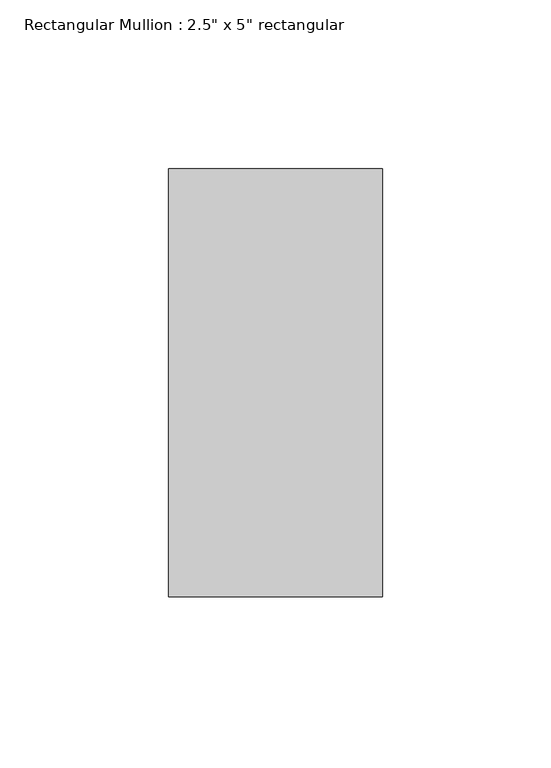
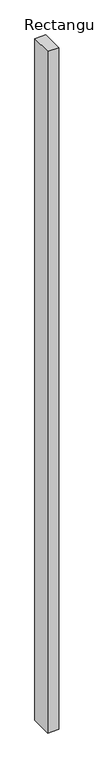
"""IFC4 building model written with IfcOpenShell, lengths in millimetres: member geometry."""

from ifc_helpers import new_model, si_unit, frame, origin, place, context, project, spatial, polyline, outline, extrude, source, transform, mapped, element, save


def member_73efc3c0(model_context):
    return source(origin(), model_context, "Body", "SweptSolid", [
        extrude(outline(polyline([(0.0, 63.5), (0.0, -63.5), (-63.5, -63.5), (-63.5, 63.5), (0.0, 63.5)])), frame((0.0, 0.0, -4163.0986763), z_axis=(0.0, 0.0, 1.0), x_axis=(1.0, 0.0, 0.0)), (0.0, 0.0, 1.0), 4163.0986763),
    ])


if __name__ == "__main__":
    model = new_model("IFC4")
    model_context = context("Model", 3, world=origin())
    ifc_project = project(units=[si_unit("LENGTHUNIT", "METRE", prefix="MILLI")], contexts=[model_context])
    site = spatial("IfcSite", under=ifc_project)
    building = spatial("IfcBuilding", under=site)
    placement = place(None, origin())
    member_shape = member_73efc3c0(model_context)
    element("IfcMember", 1, ObjectType="Rectangular Mullion : 2.5\" x 5\" rectangular", at=placement, inside=building, context=model_context, shape_type="MappedRepresentation", body=[
        mapped(member_shape, transform((0.0, 0.0, 0.0), x_axis=(1.0, 0.0, 0.0), y_axis=(0.0, 1.0, 0.0), z_axis=(0.0, 0.0, 1.0))),
    ])
    save(model, "model.ifc")

# Revit data of these elements
# Type "Rectangular Mullion : 2.5\" x 5\" rectangular"
#   built-in parameter 1007304 = 0.416667 (stored number, unit not read)
#   built-in parameter 1007301 = 0.104167 (stored number, unit not read)
#   built-in parameter 1007300 = 0.104167 (stored number, unit not read)
# Element 1 (IfcMember, "Rectangular Mullion : 2.5\" x 5\" rectangular")
#   Materials on its faces: "Aluminum"
# Materials
#   "Aluminum": class "Metal", colour RGB 247 247 247, transparency 0, Description = "Aluminum 6061", Cost = 0
